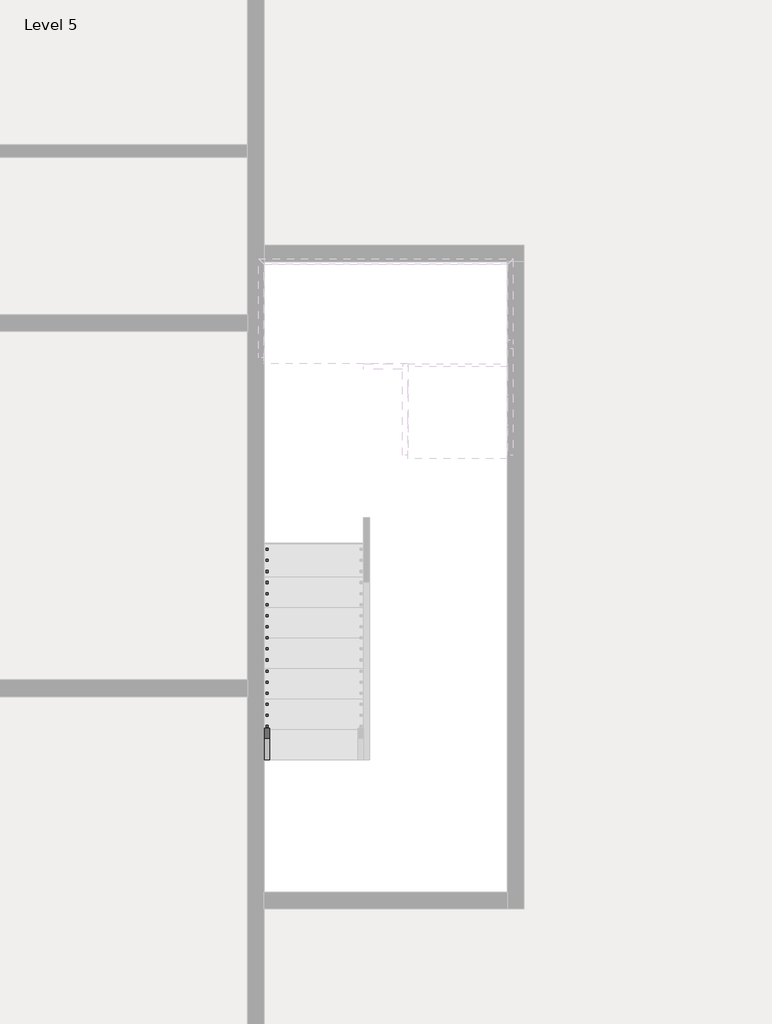
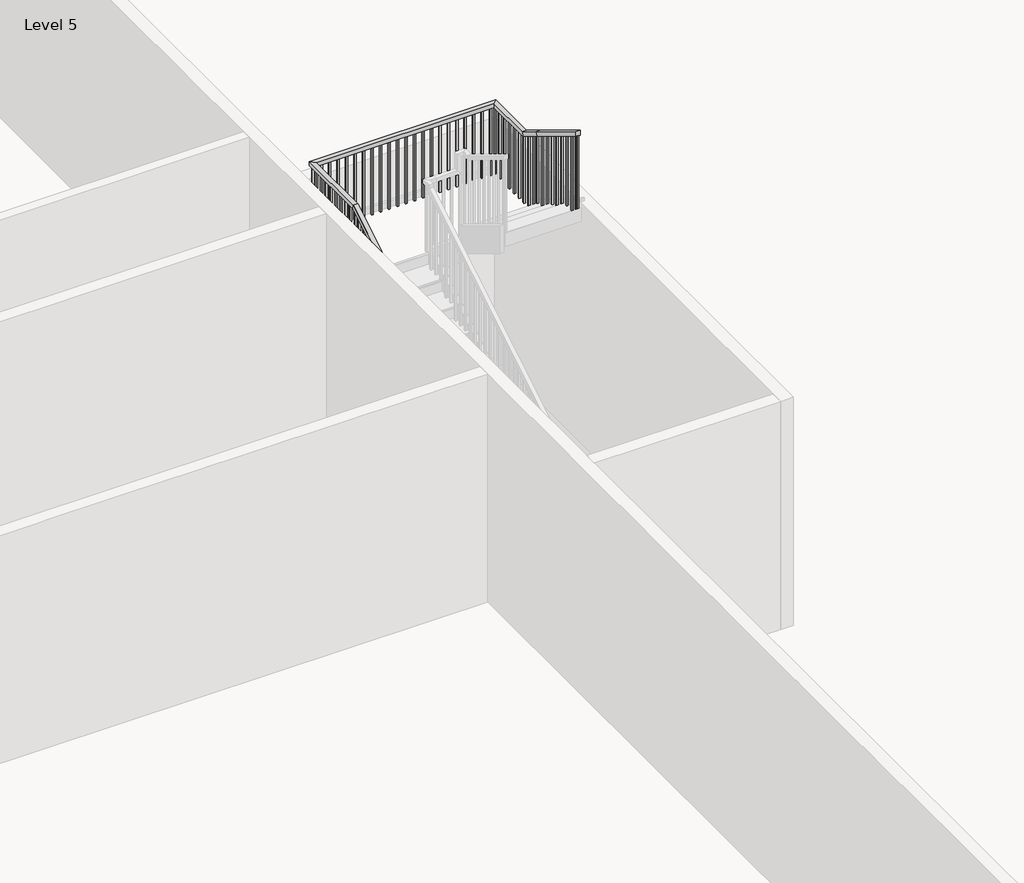
# One storey, part 6 of 8: 1 railing.
"""IFC4 building model written with IfcOpenShell, lengths in millimetres."""

from ifc_helpers import new_model, si_unit, frame, origin, place, context, project, spatial, polyline, outline, extrude, faceted_brep, element, save

model = new_model("IFC4")

# Units and contexts
model_context = context("Model", 3, world=origin())
ifc_project = project(units=[si_unit("LENGTHUNIT", "METRE", prefix="MILLI")], contexts=[model_context])

# Site, building, storey
site = spatial("IfcSite", under=ifc_project)
building = spatial("IfcBuilding", under=site)
storey = spatial("IfcBuildingStorey", under=building, Name="Level 5", Elevation=37426.6172466)

# Railing
placement = place(None, origin())
element("IfcRailing", 1, ObjectType="Handrail - Rectangular", at=placement, inside=storey, context=model_context, shape_type="SolidModel", body=[
    faceted_brep([(-3617.4415084, -23154.3851539, 38510.3505799), (-3617.4415084, -23154.3851539, 38450.9491197), (-3566.6415084, -23154.3851539, 38450.9491197), (-3566.6415084, -23154.3851539, 38510.3505799), (-3617.4415084, -19522.1851539, 40711.6839133), (-3617.4415084, -19507.9927445, 40660.8839133), (-3566.6415084, -19507.9927445, 40660.8839133), (-3566.6415084, -19522.1851539, 40711.6839133), (-3617.4415084, -18607.7851539, 40711.6839133), (-3617.4415084, -18607.7851539, 40660.8839133), (-3566.6415084, -18658.5851539, 40660.8839133), (-3566.6415084, -18658.5851539, 40711.6839133), (-1382.2415084, -18607.7851539, 40711.6839133), (-1382.2415084, -18607.7851539, 40660.8839133), (-1433.0415084, -18658.5851539, 40660.8839133), (-1433.0415084, -18658.5851539, 40711.6839133), (-1382.2415084, -19242.7851539, 40711.6839133), (-1382.2415084, -19256.9775633, 40660.8839133), (-1433.0415084, -19256.9775633, 40660.8839133), (-1433.0415084, -19242.7851539, 40711.6839133), (-1382.2415084, -19522.1851539, 40881.0172466), (-1382.2415084, -19548.5148811, 40837.5731968), (-1433.0415084, -19548.5148811, 40837.5731968), (-1433.0415084, -19522.1851539, 40881.0172466), (-1382.2415084, -20360.3851539, 41389.0172466), (-1433.0415084, -20360.3851539, 41389.0172466), (-1433.0415084, -20360.3851539, 41329.6157863), (-1382.2415084, -20360.3851539, 41329.6157863)], [[[0, 1, 2, 3]], [[1, 0, 4, 5]], [[2, 1, 5, 6]], [[3, 2, 6, 7]], [[0, 3, 7, 4]], [[5, 4, 8, 9]], [[6, 5, 9, 10]], [[7, 6, 10, 11]], [[4, 7, 11, 8]], [[9, 8, 12, 13]], [[10, 9, 13, 14]], [[11, 10, 14, 15]], [[8, 11, 15, 12]], [[13, 12, 16, 17]], [[14, 13, 17, 18]], [[15, 14, 18, 19]], [[12, 15, 19, 16]], [[17, 16, 20, 21]], [[18, 17, 21, 22]], [[19, 18, 22, 23]], [[16, 19, 23, 20]], [[24, 25, 26, 27]], [[21, 20, 24, 27]], [[22, 21, 27, 26]], [[23, 22, 26, 25]], [[20, 23, 25, 24]]]),
    extrude(outline(polyline([(-20325.4601539, 41308.4491197), (-20325.4601539, 40305.2839133), (-20344.5101539, 40305.2839133), (-20344.5101539, 41319.9945742), (-20325.4601539, 41308.4491197)])), frame((-1417.1665084, 0.0, 0.0), z_axis=(1.0, 0.0, 0.0), x_axis=(0.0, 1.0, 0.0)), (0.0, 0.0, 1.0), 19.05),
    extrude(outline(polyline([(-20223.8601539, 41246.8733621), (-20223.8601539, 40305.2839133), (-20242.9101539, 40305.2839133), (-20242.9101539, 41258.4188166), (-20223.8601539, 41246.8733621)])), frame((-1417.1665084, 0.0, 0.0), z_axis=(1.0, 0.0, 0.0), x_axis=(0.0, 1.0, 0.0)), (0.0, 0.0, 1.0), 19.05),
    extrude(outline(polyline([(-20122.2601539, 41185.2976045), (-20122.2601539, 40305.2839133), (-20141.3101539, 40305.2839133), (-20141.3101539, 41196.8430591), (-20122.2601539, 41185.2976045)])), frame((-1417.1665084, 0.0, 0.0), z_axis=(1.0, 0.0, 0.0), x_axis=(0.0, 1.0, 0.0)), (0.0, 0.0, 1.0), 19.05),
    extrude(outline(polyline([(-20020.6601539, 41123.721847), (-20020.6601539, 40135.9505799), (-20039.7101539, 40135.9505799), (-20039.7101539, 41135.2673015), (-20020.6601539, 41123.721847)])), frame((-1417.1665084, 0.0, 0.0), z_axis=(1.0, 0.0, 0.0), x_axis=(0.0, 1.0, 0.0)), (0.0, 0.0, 1.0), 19.05),
    extrude(outline(polyline([(-19919.0601539, 41062.1460894), (-19919.0601539, 40135.9505799), (-19938.1101539, 40135.9505799), (-19938.1101539, 41073.6915439), (-19919.0601539, 41062.1460894)])), frame((-1417.1665084, 0.0, 0.0), z_axis=(1.0, 0.0, 0.0), x_axis=(0.0, 1.0, 0.0)), (0.0, 0.0, 1.0), 19.05),
    extrude(outline(polyline([(-19817.4601539, 41000.5703318), (-19817.4601539, 40135.9505799), (-19836.5101539, 40135.9505799), (-19836.5101539, 41012.1157863), (-19817.4601539, 41000.5703318)])), frame((-1417.1665084, 0.0, 0.0), z_axis=(1.0, 0.0, 0.0), x_axis=(0.0, 1.0, 0.0)), (0.0, 0.0, 1.0), 19.05),
    extrude(outline(polyline([(-19715.8601539, 40938.9945742), (-19715.8601539, 39966.6172466), (-19734.9101539, 39966.6172466), (-19734.9101539, 40950.5400288), (-19715.8601539, 40938.9945742)])), frame((-1417.1665084, 0.0, 0.0), z_axis=(1.0, 0.0, 0.0), x_axis=(0.0, 1.0, 0.0)), (0.0, 0.0, 1.0), 19.05),
    extrude(outline(polyline([(-19614.2601539, 40877.4188166), (-19614.2601539, 39966.6172466), (-19633.3101539, 39966.6172466), (-19633.3101539, 40888.9642712), (-19614.2601539, 40877.4188166)])), frame((-1417.1665084, 0.0, 0.0), z_axis=(1.0, 0.0, 0.0), x_axis=(0.0, 1.0, 0.0)), (0.0, 0.0, 1.0), 19.05),
    extrude(outline(polyline([(-19436.4601539, 40769.6612409), (-19436.4601539, 39797.2839133), (-19455.5101539, 39797.2839133), (-19455.5101539, 40781.2066954), (-19436.4601539, 40769.6612409)])), frame((-1417.1665084, 0.0, 0.0), z_axis=(1.0, 0.0, 0.0), x_axis=(0.0, 1.0, 0.0)), (0.0, 0.0, 1.0), 19.05),
    extrude(outline(polyline([(-19334.8601539, 40708.0854833), (-19334.8601539, 39797.2839133), (-19353.9101539, 39797.2839133), (-19353.9101539, 40719.6309379), (-19334.8601539, 40708.0854833)])), frame((-1417.1665084, 0.0, 0.0), z_axis=(1.0, 0.0, 0.0), x_axis=(0.0, 1.0, 0.0)), (0.0, 0.0, 1.0), 19.05),
    extrude(outline(polyline([(-1398.1165084, -19233.2601539), (-1398.1165084, -19252.3101539), (-1417.1665084, -19252.3101539), (-1417.1665084, -19233.2601539), (-1398.1165084, -19233.2601539)])), frame((0.0, 0.0, 39797.2839133), z_axis=(0.0, 0.0, 1.0), x_axis=(1.0, 0.0, 0.0)), (0.0, 0.0, 1.0), 863.6),
    extrude(outline(polyline([(-1398.1165084, -19131.6601539), (-1398.1165084, -19150.7101539), (-1417.1665084, -19150.7101539), (-1417.1665084, -19131.6601539), (-1398.1165084, -19131.6601539)])), frame((0.0, 0.0, 39797.2839133), z_axis=(0.0, 0.0, 1.0), x_axis=(1.0, 0.0, 0.0)), (0.0, 0.0, 1.0), 863.6),
    extrude(outline(polyline([(-1398.1165084, -19030.0601539), (-1398.1165084, -19049.1101539), (-1417.1665084, -19049.1101539), (-1417.1665084, -19030.0601539), (-1398.1165084, -19030.0601539)])), frame((0.0, 0.0, 39797.2839133), z_axis=(0.0, 0.0, 1.0), x_axis=(1.0, 0.0, 0.0)), (0.0, 0.0, 1.0), 863.6),
    extrude(outline(polyline([(-1398.1165084, -18928.4601539), (-1398.1165084, -18947.5101539), (-1417.1665084, -18947.5101539), (-1417.1665084, -18928.4601539), (-1398.1165084, -18928.4601539)])), frame((0.0, 0.0, 39797.2839133), z_axis=(0.0, 0.0, 1.0), x_axis=(1.0, 0.0, 0.0)), (0.0, 0.0, 1.0), 863.6),
    extrude(outline(polyline([(-1398.1165084, -18826.8601539), (-1398.1165084, -18845.9101539), (-1417.1665084, -18845.9101539), (-1417.1665084, -18826.8601539), (-1398.1165084, -18826.8601539)])), frame((0.0, 0.0, 39797.2839133), z_axis=(0.0, 0.0, 1.0), x_axis=(1.0, 0.0, 0.0)), (0.0, 0.0, 1.0), 863.6),
    extrude(outline(polyline([(-1398.1165084, -18725.2601539), (-1398.1165084, -18744.3101539), (-1417.1665084, -18744.3101539), (-1417.1665084, -18725.2601539), (-1398.1165084, -18725.2601539)])), frame((0.0, 0.0, 39797.2839133), z_axis=(0.0, 0.0, 1.0), x_axis=(1.0, 0.0, 0.0)), (0.0, 0.0, 1.0), 863.6),
    extrude(outline(polyline([(-1467.9665084, -18623.6601539), (-1448.9165084, -18623.6601539), (-1448.9165084, -18642.7101539), (-1467.9665084, -18642.7101539), (-1467.9665084, -18623.6601539)])), frame((0.0, 0.0, 39797.2839133), z_axis=(0.0, 0.0, 1.0), x_axis=(1.0, 0.0, 0.0)), (0.0, 0.0, 1.0), 863.6),
    extrude(outline(polyline([(-1569.5665084, -18623.6601539), (-1550.5165084, -18623.6601539), (-1550.5165084, -18642.7101539), (-1569.5665084, -18642.7101539), (-1569.5665084, -18623.6601539)])), frame((0.0, 0.0, 39797.2839133), z_axis=(0.0, 0.0, 1.0), x_axis=(1.0, 0.0, 0.0)), (0.0, 0.0, 1.0), 863.6),
    extrude(outline(polyline([(-1671.1665084, -18623.6601539), (-1652.1165084, -18623.6601539), (-1652.1165084, -18642.7101539), (-1671.1665084, -18642.7101539), (-1671.1665084, -18623.6601539)])), frame((0.0, 0.0, 39797.2839133), z_axis=(0.0, 0.0, 1.0), x_axis=(1.0, 0.0, 0.0)), (0.0, 0.0, 1.0), 863.6),
    extrude(outline(polyline([(-1772.7665084, -18623.6601539), (-1753.7165084, -18623.6601539), (-1753.7165084, -18642.7101539), (-1772.7665084, -18642.7101539), (-1772.7665084, -18623.6601539)])), frame((0.0, 0.0, 39797.2839133), z_axis=(0.0, 0.0, 1.0), x_axis=(1.0, 0.0, 0.0)), (0.0, 0.0, 1.0), 863.6),
    extrude(outline(polyline([(-1874.3665084, -18623.6601539), (-1855.3165084, -18623.6601539), (-1855.3165084, -18642.7101539), (-1874.3665084, -18642.7101539), (-1874.3665084, -18623.6601539)])), frame((0.0, 0.0, 39797.2839133), z_axis=(0.0, 0.0, 1.0), x_axis=(1.0, 0.0, 0.0)), (0.0, 0.0, 1.0), 863.6),
    extrude(outline(polyline([(-1975.9665084, -18623.6601539), (-1956.9165084, -18623.6601539), (-1956.9165084, -18642.7101539), (-1975.9665084, -18642.7101539), (-1975.9665084, -18623.6601539)])), frame((0.0, 0.0, 39797.2839133), z_axis=(0.0, 0.0, 1.0), x_axis=(1.0, 0.0, 0.0)), (0.0, 0.0, 1.0), 863.6),
    extrude(outline(polyline([(-2077.5665084, -18623.6601539), (-2058.5165084, -18623.6601539), (-2058.5165084, -18642.7101539), (-2077.5665084, -18642.7101539), (-2077.5665084, -18623.6601539)])), frame((0.0, 0.0, 39797.2839133), z_axis=(0.0, 0.0, 1.0), x_axis=(1.0, 0.0, 0.0)), (0.0, 0.0, 1.0), 863.6),
    extrude(outline(polyline([(-2179.1665084, -18623.6601539), (-2160.1165084, -18623.6601539), (-2160.1165084, -18642.7101539), (-2179.1665084, -18642.7101539), (-2179.1665084, -18623.6601539)])), frame((0.0, 0.0, 39797.2839133), z_axis=(0.0, 0.0, 1.0), x_axis=(1.0, 0.0, 0.0)), (0.0, 0.0, 1.0), 863.6),
    extrude(outline(polyline([(-2280.7665084, -18623.6601539), (-2261.7165084, -18623.6601539), (-2261.7165084, -18642.7101539), (-2280.7665084, -18642.7101539), (-2280.7665084, -18623.6601539)])), frame((0.0, 0.0, 39797.2839133), z_axis=(0.0, 0.0, 1.0), x_axis=(1.0, 0.0, 0.0)), (0.0, 0.0, 1.0), 863.6),
    extrude(outline(polyline([(-2382.3665084, -18623.6601539), (-2363.3165084, -18623.6601539), (-2363.3165084, -18642.7101539), (-2382.3665084, -18642.7101539), (-2382.3665084, -18623.6601539)])), frame((0.0, 0.0, 39797.2839133), z_axis=(0.0, 0.0, 1.0), x_axis=(1.0, 0.0, 0.0)), (0.0, 0.0, 1.0), 863.6),
    extrude(outline(polyline([(-2483.9665084, -18623.6601539), (-2464.9165084, -18623.6601539), (-2464.9165084, -18642.7101539), (-2483.9665084, -18642.7101539), (-2483.9665084, -18623.6601539)])), frame((0.0, 0.0, 39797.2839133), z_axis=(0.0, 0.0, 1.0), x_axis=(1.0, 0.0, 0.0)), (0.0, 0.0, 1.0), 863.6),
    extrude(outline(polyline([(-2585.5665084, -18623.6601539), (-2566.5165084, -18623.6601539), (-2566.5165084, -18642.7101539), (-2585.5665084, -18642.7101539), (-2585.5665084, -18623.6601539)])), frame((0.0, 0.0, 39797.2839133), z_axis=(0.0, 0.0, 1.0), x_axis=(1.0, 0.0, 0.0)), (0.0, 0.0, 1.0), 863.6),
    extrude(outline(polyline([(-2687.1665084, -18623.6601539), (-2668.1165084, -18623.6601539), (-2668.1165084, -18642.7101539), (-2687.1665084, -18642.7101539), (-2687.1665084, -18623.6601539)])), frame((0.0, 0.0, 39797.2839133), z_axis=(0.0, 0.0, 1.0), x_axis=(1.0, 0.0, 0.0)), (0.0, 0.0, 1.0), 863.6),
    extrude(outline(polyline([(-2788.7665084, -18623.6601539), (-2769.7165084, -18623.6601539), (-2769.7165084, -18642.7101539), (-2788.7665084, -18642.7101539), (-2788.7665084, -18623.6601539)])), frame((0.0, 0.0, 39797.2839133), z_axis=(0.0, 0.0, 1.0), x_axis=(1.0, 0.0, 0.0)), (0.0, 0.0, 1.0), 863.6),
    extrude(outline(polyline([(-2890.3665084, -18623.6601539), (-2871.3165084, -18623.6601539), (-2871.3165084, -18642.7101539), (-2890.3665084, -18642.7101539), (-2890.3665084, -18623.6601539)])), frame((0.0, 0.0, 39797.2839133), z_axis=(0.0, 0.0, 1.0), x_axis=(1.0, 0.0, 0.0)), (0.0, 0.0, 1.0), 863.6),
    extrude(outline(polyline([(-2991.9665084, -18623.6601539), (-2972.9165084, -18623.6601539), (-2972.9165084, -18642.7101539), (-2991.9665084, -18642.7101539), (-2991.9665084, -18623.6601539)])), frame((0.0, 0.0, 39797.2839133), z_axis=(0.0, 0.0, 1.0), x_axis=(1.0, 0.0, 0.0)), (0.0, 0.0, 1.0), 863.6),
    extrude(outline(polyline([(-3093.5665084, -18623.6601539), (-3074.5165084, -18623.6601539), (-3074.5165084, -18642.7101539), (-3093.5665084, -18642.7101539), (-3093.5665084, -18623.6601539)])), frame((0.0, 0.0, 39797.2839133), z_axis=(0.0, 0.0, 1.0), x_axis=(1.0, 0.0, 0.0)), (0.0, 0.0, 1.0), 863.6),
    extrude(outline(polyline([(-3195.1665084, -18623.6601539), (-3176.1165084, -18623.6601539), (-3176.1165084, -18642.7101539), (-3195.1665084, -18642.7101539), (-3195.1665084, -18623.6601539)])), frame((0.0, 0.0, 39797.2839133), z_axis=(0.0, 0.0, 1.0), x_axis=(1.0, 0.0, 0.0)), (0.0, 0.0, 1.0), 863.6),
    extrude(outline(polyline([(-3296.7665084, -18623.6601539), (-3277.7165084, -18623.6601539), (-3277.7165084, -18642.7101539), (-3296.7665084, -18642.7101539), (-3296.7665084, -18623.6601539)])), frame((0.0, 0.0, 39797.2839133), z_axis=(0.0, 0.0, 1.0), x_axis=(1.0, 0.0, 0.0)), (0.0, 0.0, 1.0), 863.6),
    extrude(outline(polyline([(-3398.3665084, -18623.6601539), (-3379.3165084, -18623.6601539), (-3379.3165084, -18642.7101539), (-3398.3665084, -18642.7101539), (-3398.3665084, -18623.6601539)])), frame((0.0, 0.0, 39797.2839133), z_axis=(0.0, 0.0, 1.0), x_axis=(1.0, 0.0, 0.0)), (0.0, 0.0, 1.0), 863.6),
    extrude(outline(polyline([(-3499.9665084, -18623.6601539), (-3480.9165084, -18623.6601539), (-3480.9165084, -18642.7101539), (-3499.9665084, -18642.7101539), (-3499.9665084, -18623.6601539)])), frame((0.0, 0.0, 39797.2839133), z_axis=(0.0, 0.0, 1.0), x_axis=(1.0, 0.0, 0.0)), (0.0, 0.0, 1.0), 863.6),
    extrude(outline(polyline([(-3601.5665084, -18718.9101539), (-3601.5665084, -18699.8601539), (-3582.5165084, -18699.8601539), (-3582.5165084, -18718.9101539), (-3601.5665084, -18718.9101539)])), frame((0.0, 0.0, 39797.2839133), z_axis=(0.0, 0.0, 1.0), x_axis=(1.0, 0.0, 0.0)), (0.0, 0.0, 1.0), 863.6),
    extrude(outline(polyline([(-3601.5665084, -18820.5101539), (-3601.5665084, -18801.4601539), (-3582.5165084, -18801.4601539), (-3582.5165084, -18820.5101539), (-3601.5665084, -18820.5101539)])), frame((0.0, 0.0, 39797.2839133), z_axis=(0.0, 0.0, 1.0), x_axis=(1.0, 0.0, 0.0)), (0.0, 0.0, 1.0), 863.6),
    extrude(outline(polyline([(-3601.5665084, -18922.1101539), (-3601.5665084, -18903.0601539), (-3582.5165084, -18903.0601539), (-3582.5165084, -18922.1101539), (-3601.5665084, -18922.1101539)])), frame((0.0, 0.0, 39797.2839133), z_axis=(0.0, 0.0, 1.0), x_axis=(1.0, 0.0, 0.0)), (0.0, 0.0, 1.0), 863.6),
    extrude(outline(polyline([(-3601.5665084, -19023.7101539), (-3601.5665084, -19004.6601539), (-3582.5165084, -19004.6601539), (-3582.5165084, -19023.7101539), (-3601.5665084, -19023.7101539)])), frame((0.0, 0.0, 39797.2839133), z_axis=(0.0, 0.0, 1.0), x_axis=(1.0, 0.0, 0.0)), (0.0, 0.0, 1.0), 863.6),
    extrude(outline(polyline([(-3601.5665084, -19125.3101539), (-3601.5665084, -19106.2601539), (-3582.5165084, -19106.2601539), (-3582.5165084, -19125.3101539), (-3601.5665084, -19125.3101539)])), frame((0.0, 0.0, 39797.2839133), z_axis=(0.0, 0.0, 1.0), x_axis=(1.0, 0.0, 0.0)), (0.0, 0.0, 1.0), 863.6),
    extrude(outline(polyline([(-3601.5665084, -19226.9101539), (-3601.5665084, -19207.8601539), (-3582.5165084, -19207.8601539), (-3582.5165084, -19226.9101539), (-3601.5665084, -19226.9101539)])), frame((0.0, 0.0, 39797.2839133), z_axis=(0.0, 0.0, 1.0), x_axis=(1.0, 0.0, 0.0)), (0.0, 0.0, 1.0), 863.6),
    extrude(outline(polyline([(-3601.5665084, -19328.5101539), (-3601.5665084, -19309.4601539), (-3582.5165084, -19309.4601539), (-3582.5165084, -19328.5101539), (-3601.5665084, -19328.5101539)])), frame((0.0, 0.0, 39797.2839133), z_axis=(0.0, 0.0, 1.0), x_axis=(1.0, 0.0, 0.0)), (0.0, 0.0, 1.0), 863.6),
    extrude(outline(polyline([(-3601.5665084, -19430.1101539), (-3601.5665084, -19411.0601539), (-3582.5165084, -19411.0601539), (-3582.5165084, -19430.1101539), (-3601.5665084, -19430.1101539)])), frame((0.0, 0.0, 39797.2839133), z_axis=(0.0, 0.0, 1.0), x_axis=(1.0, 0.0, 0.0)), (0.0, 0.0, 1.0), 863.6),
    extrude(outline(polyline([(-19588.8601539, 40611.8733621), (-19588.8601539, 39627.9505799), (-19607.9101539, 39627.9505799), (-19607.9101539, 40600.3279076), (-19588.8601539, 40611.8733621)])), frame((-3601.5665084, 0.0, 0.0), z_axis=(1.0, 0.0, 0.0), x_axis=(0.0, 1.0, 0.0)), (0.0, 0.0, 1.0), 19.05),
    extrude(outline(polyline([(-19690.4601539, 40550.2976045), (-19690.4601539, 39627.9505799), (-19709.5101539, 39627.9505799), (-19709.5101539, 40538.75215), (-19690.4601539, 40550.2976045)])), frame((-3601.5665084, 0.0, 0.0), z_axis=(1.0, 0.0, 0.0), x_axis=(0.0, 1.0, 0.0)), (0.0, 0.0, 1.0), 19.05),
    extrude(outline(polyline([(-19792.0601539, 40488.721847), (-19792.0601539, 39627.9505799), (-19811.1101539, 39627.9505799), (-19811.1101539, 40477.1763924), (-19792.0601539, 40488.721847)])), frame((-3601.5665084, 0.0, 0.0), z_axis=(1.0, 0.0, 0.0), x_axis=(0.0, 1.0, 0.0)), (0.0, 0.0, 1.0), 19.05),
    extrude(outline(polyline([(-19893.6601539, 40427.1460894), (-19893.6601539, 39458.6172466), (-19912.7101539, 39458.6172466), (-19912.7101539, 40415.6006348), (-19893.6601539, 40427.1460894)])), frame((-3601.5665084, 0.0, 0.0), z_axis=(1.0, 0.0, 0.0), x_axis=(0.0, 1.0, 0.0)), (0.0, 0.0, 1.0), 19.05),
    extrude(outline(polyline([(-19995.2601539, 40365.5703318), (-19995.2601539, 39458.6172466), (-20014.3101539, 39458.6172466), (-20014.3101539, 40354.0248773), (-19995.2601539, 40365.5703318)])), frame((-3601.5665084, 0.0, 0.0), z_axis=(1.0, 0.0, 0.0), x_axis=(0.0, 1.0, 0.0)), (0.0, 0.0, 1.0), 19.05),
    extrude(outline(polyline([(-20096.8601539, 40303.9945742), (-20096.8601539, 39289.2839133), (-20115.9101539, 39289.2839133), (-20115.9101539, 40292.4491197), (-20096.8601539, 40303.9945742)])), frame((-3601.5665084, 0.0, 0.0), z_axis=(1.0, 0.0, 0.0), x_axis=(0.0, 1.0, 0.0)), (0.0, 0.0, 1.0), 19.05),
    extrude(outline(polyline([(-20198.4601539, 40242.4188166), (-20198.4601539, 39289.2839133), (-20217.5101539, 39289.2839133), (-20217.5101539, 40230.8733621), (-20198.4601539, 40242.4188166)])), frame((-3601.5665084, 0.0, 0.0), z_axis=(1.0, 0.0, 0.0), x_axis=(0.0, 1.0, 0.0)), (0.0, 0.0, 1.0), 19.05),
    extrude(outline(polyline([(-20300.0601539, 40180.8430591), (-20300.0601539, 39289.2839133), (-20319.1101539, 39289.2839133), (-20319.1101539, 40169.2976045), (-20300.0601539, 40180.8430591)])), frame((-3601.5665084, 0.0, 0.0), z_axis=(1.0, 0.0, 0.0), x_axis=(0.0, 1.0, 0.0)), (0.0, 0.0, 1.0), 19.05),
    extrude(outline(polyline([(-20401.6601539, 40119.2673015), (-20401.6601539, 39119.9505799), (-20420.7101539, 39119.9505799), (-20420.7101539, 40107.721847), (-20401.6601539, 40119.2673015)])), frame((-3601.5665084, 0.0, 0.0), z_axis=(1.0, 0.0, 0.0), x_axis=(0.0, 1.0, 0.0)), (0.0, 0.0, 1.0), 19.05),
    extrude(outline(polyline([(-20503.2601539, 40057.6915439), (-20503.2601539, 39119.9505799), (-20522.3101539, 39119.9505799), (-20522.3101539, 40046.1460894), (-20503.2601539, 40057.6915439)])), frame((-3601.5665084, 0.0, 0.0), z_axis=(1.0, 0.0, 0.0), x_axis=(0.0, 1.0, 0.0)), (0.0, 0.0, 1.0), 19.05),
    extrude(outline(polyline([(-20604.8601539, 39996.1157863), (-20604.8601539, 39119.9505799), (-20623.9101539, 39119.9505799), (-20623.9101539, 39984.5703318), (-20604.8601539, 39996.1157863)])), frame((-3601.5665084, 0.0, 0.0), z_axis=(1.0, 0.0, 0.0), x_axis=(0.0, 1.0, 0.0)), (0.0, 0.0, 1.0), 19.05),
    extrude(outline(polyline([(-20706.4601539, 39934.5400288), (-20706.4601539, 38950.6172466), (-20725.5101539, 38950.6172466), (-20725.5101539, 39922.9945742), (-20706.4601539, 39934.5400288)])), frame((-3601.5665084, 0.0, 0.0), z_axis=(1.0, 0.0, 0.0), x_axis=(0.0, 1.0, 0.0)), (0.0, 0.0, 1.0), 19.05),
    extrude(outline(polyline([(-20808.0601539, 39872.9642712), (-20808.0601539, 38950.6172466), (-20827.1101539, 38950.6172466), (-20827.1101539, 39861.4188166), (-20808.0601539, 39872.9642712)])), frame((-3601.5665084, 0.0, 0.0), z_axis=(1.0, 0.0, 0.0), x_axis=(0.0, 1.0, 0.0)), (0.0, 0.0, 1.0), 19.05),
    extrude(outline(polyline([(-20909.6601539, 39811.3885136), (-20909.6601539, 38950.6172466), (-20928.7101539, 38950.6172466), (-20928.7101539, 39799.8430591), (-20909.6601539, 39811.3885136)])), frame((-3601.5665084, 0.0, 0.0), z_axis=(1.0, 0.0, 0.0), x_axis=(0.0, 1.0, 0.0)), (0.0, 0.0, 1.0), 19.05),
    extrude(outline(polyline([(-21011.2601539, 39749.812756), (-21011.2601539, 38781.2839133), (-21030.3101539, 38781.2839133), (-21030.3101539, 39738.2673015), (-21011.2601539, 39749.812756)])), frame((-3601.5665084, 0.0, 0.0), z_axis=(1.0, 0.0, 0.0), x_axis=(0.0, 1.0, 0.0)), (0.0, 0.0, 1.0), 19.05),
    extrude(outline(polyline([(-21112.8601539, 39688.2369985), (-21112.8601539, 38781.2839133), (-21131.9101539, 38781.2839133), (-21131.9101539, 39676.6915439), (-21112.8601539, 39688.2369985)])), frame((-3601.5665084, 0.0, 0.0), z_axis=(1.0, 0.0, 0.0), x_axis=(0.0, 1.0, 0.0)), (0.0, 0.0, 1.0), 19.05),
    extrude(outline(polyline([(-21214.4601539, 39626.6612409), (-21214.4601539, 38611.9505799), (-21233.5101539, 38611.9505799), (-21233.5101539, 39615.1157863), (-21214.4601539, 39626.6612409)])), frame((-3601.5665084, 0.0, 0.0), z_axis=(1.0, 0.0, 0.0), x_axis=(0.0, 1.0, 0.0)), (0.0, 0.0, 1.0), 19.05),
    extrude(outline(polyline([(-21316.0601539, 39565.0854833), (-21316.0601539, 38611.9505799), (-21335.1101539, 38611.9505799), (-21335.1101539, 39553.5400288), (-21316.0601539, 39565.0854833)])), frame((-3601.5665084, 0.0, 0.0), z_axis=(1.0, 0.0, 0.0), x_axis=(0.0, 1.0, 0.0)), (0.0, 0.0, 1.0), 19.05),
    extrude(outline(polyline([(-21417.6601539, 39503.5097257), (-21417.6601539, 38611.9505799), (-21436.7101539, 38611.9505799), (-21436.7101539, 39491.9642712), (-21417.6601539, 39503.5097257)])), frame((-3601.5665084, 0.0, 0.0), z_axis=(1.0, 0.0, 0.0), x_axis=(0.0, 1.0, 0.0)), (0.0, 0.0, 1.0), 19.05),
    extrude(outline(polyline([(-21519.2601539, 39441.9339682), (-21519.2601539, 38442.6172466), (-21538.3101539, 38442.6172466), (-21538.3101539, 39430.3885136), (-21519.2601539, 39441.9339682)])), frame((-3601.5665084, 0.0, 0.0), z_axis=(1.0, 0.0, 0.0), x_axis=(0.0, 1.0, 0.0)), (0.0, 0.0, 1.0), 19.05),
    extrude(outline(polyline([(-21620.8601539, 39380.3582106), (-21620.8601539, 38442.6172466), (-21639.9101539, 38442.6172466), (-21639.9101539, 39368.812756), (-21620.8601539, 39380.3582106)])), frame((-3601.5665084, 0.0, 0.0), z_axis=(1.0, 0.0, 0.0), x_axis=(0.0, 1.0, 0.0)), (0.0, 0.0, 1.0), 19.05),
    extrude(outline(polyline([(-21722.4601539, 39318.782453), (-21722.4601539, 38442.6172466), (-21741.5101539, 38442.6172466), (-21741.5101539, 39307.2369985), (-21722.4601539, 39318.782453)])), frame((-3601.5665084, 0.0, 0.0), z_axis=(1.0, 0.0, 0.0), x_axis=(0.0, 1.0, 0.0)), (0.0, 0.0, 1.0), 19.05),
    extrude(outline(polyline([(-21824.0601539, 39257.2066954), (-21824.0601539, 38273.2839133), (-21843.1101539, 38273.2839133), (-21843.1101539, 39245.6612409), (-21824.0601539, 39257.2066954)])), frame((-3601.5665084, 0.0, 0.0), z_axis=(1.0, 0.0, 0.0), x_axis=(0.0, 1.0, 0.0)), (0.0, 0.0, 1.0), 19.05),
    extrude(outline(polyline([(-21925.6601539, 39195.6309379), (-21925.6601539, 38273.2839133), (-21944.7101539, 38273.2839133), (-21944.7101539, 39184.0854833), (-21925.6601539, 39195.6309379)])), frame((-3601.5665084, 0.0, 0.0), z_axis=(1.0, 0.0, 0.0), x_axis=(0.0, 1.0, 0.0)), (0.0, 0.0, 1.0), 19.05),
    extrude(outline(polyline([(-22027.2601539, 39134.0551803), (-22027.2601539, 38273.2839133), (-22046.3101539, 38273.2839133), (-22046.3101539, 39122.5097257), (-22027.2601539, 39134.0551803)])), frame((-3601.5665084, 0.0, 0.0), z_axis=(1.0, 0.0, 0.0), x_axis=(0.0, 1.0, 0.0)), (0.0, 0.0, 1.0), 19.05),
    extrude(outline(polyline([(-22128.8601539, 39072.4794227), (-22128.8601539, 38103.9505799), (-22147.9101539, 38103.9505799), (-22147.9101539, 39060.9339682), (-22128.8601539, 39072.4794227)])), frame((-3601.5665084, 0.0, 0.0), z_axis=(1.0, 0.0, 0.0), x_axis=(0.0, 1.0, 0.0)), (0.0, 0.0, 1.0), 19.05),
    extrude(outline(polyline([(-22230.4601539, 39010.9036651), (-22230.4601539, 38103.9505799), (-22249.5101539, 38103.9505799), (-22249.5101539, 38999.3582106), (-22230.4601539, 39010.9036651)])), frame((-3601.5665084, 0.0, 0.0), z_axis=(1.0, 0.0, 0.0), x_axis=(0.0, 1.0, 0.0)), (0.0, 0.0, 1.0), 19.05),
    extrude(outline(polyline([(-22332.0601539, 38949.3279076), (-22332.0601539, 37934.6172466), (-22351.1101539, 37934.6172466), (-22351.1101539, 38937.782453), (-22332.0601539, 38949.3279076)])), frame((-3601.5665084, 0.0, 0.0), z_axis=(1.0, 0.0, 0.0), x_axis=(0.0, 1.0, 0.0)), (0.0, 0.0, 1.0), 19.05),
    extrude(outline(polyline([(-22433.6601539, 38887.75215), (-22433.6601539, 37934.6172466), (-22452.7101539, 37934.6172466), (-22452.7101539, 38876.2066954), (-22433.6601539, 38887.75215)])), frame((-3601.5665084, 0.0, 0.0), z_axis=(1.0, 0.0, 0.0), x_axis=(0.0, 1.0, 0.0)), (0.0, 0.0, 1.0), 19.05),
    extrude(outline(polyline([(-22535.2601539, 38826.1763924), (-22535.2601539, 37934.6172466), (-22554.3101539, 37934.6172466), (-22554.3101539, 38814.6309379), (-22535.2601539, 38826.1763924)])), frame((-3601.5665084, 0.0, 0.0), z_axis=(1.0, 0.0, 0.0), x_axis=(0.0, 1.0, 0.0)), (0.0, 0.0, 1.0), 19.05),
    extrude(outline(polyline([(-22636.8601539, 38764.6006348), (-22636.8601539, 37765.2839133), (-22655.9101539, 37765.2839133), (-22655.9101539, 38753.0551803), (-22636.8601539, 38764.6006348)])), frame((-3601.5665084, 0.0, 0.0), z_axis=(1.0, 0.0, 0.0), x_axis=(0.0, 1.0, 0.0)), (0.0, 0.0, 1.0), 19.05),
    extrude(outline(polyline([(-22738.4601539, 38703.0248773), (-22738.4601539, 37765.2839133), (-22757.5101539, 37765.2839133), (-22757.5101539, 38691.4794227), (-22738.4601539, 38703.0248773)])), frame((-3601.5665084, 0.0, 0.0), z_axis=(1.0, 0.0, 0.0), x_axis=(0.0, 1.0, 0.0)), (0.0, 0.0, 1.0), 19.05),
    extrude(outline(polyline([(-22840.0601539, 38641.4491197), (-22840.0601539, 37765.2839133), (-22859.1101539, 37765.2839133), (-22859.1101539, 38629.9036651), (-22840.0601539, 38641.4491197)])), frame((-3601.5665084, 0.0, 0.0), z_axis=(1.0, 0.0, 0.0), x_axis=(0.0, 1.0, 0.0)), (0.0, 0.0, 1.0), 19.05),
    extrude(outline(polyline([(-22941.6601539, 38579.8733621), (-22941.6601539, 37595.9505799), (-22960.7101539, 37595.9505799), (-22960.7101539, 38568.3279076), (-22941.6601539, 38579.8733621)])), frame((-3601.5665084, 0.0, 0.0), z_axis=(1.0, 0.0, 0.0), x_axis=(0.0, 1.0, 0.0)), (0.0, 0.0, 1.0), 19.05),
    extrude(outline(polyline([(-23043.2601539, 38518.2976045), (-23043.2601539, 37595.9505799), (-23062.3101539, 37595.9505799), (-23062.3101539, 38506.75215), (-23043.2601539, 38518.2976045)])), frame((-3601.5665084, 0.0, 0.0), z_axis=(1.0, 0.0, 0.0), x_axis=(0.0, 1.0, 0.0)), (0.0, 0.0, 1.0), 19.05),
    extrude(outline(polyline([(-19512.6601539, 40815.8430591), (-19512.6601539, 39797.2839133), (-19531.7101539, 39797.2839133), (-19531.7101539, 40827.3885136), (-19512.6601539, 40815.8430591)])), frame((-1417.1665084, 0.0, 0.0), z_axis=(1.0, 0.0, 0.0), x_axis=(0.0, 1.0, 0.0)), (0.0, 0.0, 1.0), 19.05),
    extrude(outline(polyline([(-1417.1665084, -18623.6601539), (-1398.1165084, -18623.6601539), (-1398.1165084, -18642.7101539), (-1417.1665084, -18642.7101539), (-1417.1665084, -18623.6601539)])), frame((0.0, 0.0, 39797.2839133), z_axis=(0.0, 0.0, 1.0), x_axis=(1.0, 0.0, 0.0)), (0.0, 0.0, 1.0), 863.6),
    extrude(outline(polyline([(-3601.5665084, -18642.7101539), (-3601.5665084, -18623.6601539), (-3582.5165084, -18623.6601539), (-3582.5165084, -18642.7101539), (-3601.5665084, -18642.7101539)])), frame((0.0, 0.0, 39797.2839133), z_axis=(0.0, 0.0, 1.0), x_axis=(1.0, 0.0, 0.0)), (0.0, 0.0, 1.0), 863.6),
    extrude(outline(polyline([(-19512.6601539, 40658.0551803), (-19512.6601539, 39797.2839133), (-19531.7101539, 39797.2839133), (-19531.7101539, 40646.5097257), (-19512.6601539, 40658.0551803)])), frame((-3601.5665084, 0.0, 0.0), z_axis=(1.0, 0.0, 0.0), x_axis=(0.0, 1.0, 0.0)), (0.0, 0.0, 1.0), 19.05),
    extrude(outline(polyline([(-20341.3351539, 41318.0703318), (-20341.3351539, 40305.2839133), (-20360.3851539, 40305.2839133), (-20360.3851539, 41329.6157863), (-20341.3351539, 41318.0703318)])), frame((-1417.1665084, 0.0, 0.0), z_axis=(1.0, 0.0, 0.0), x_axis=(0.0, 1.0, 0.0)), (0.0, 0.0, 1.0), 19.05),
    extrude(outline(polyline([(-23135.3351539, 38462.4945742), (-23135.3351539, 37595.9505799), (-23154.3851539, 37595.9505799), (-23154.3851539, 38450.9491197), (-23135.3351539, 38462.4945742)])), frame((-3601.5665084, 0.0, 0.0), z_axis=(1.0, 0.0, 0.0), x_axis=(0.0, 1.0, 0.0)), (0.0, 0.0, 1.0), 19.05),
])

save(model, "model.ifc")

# Revit data of these elements
# Type "Handrail - Rectangular"
#   Assembly Code = "C2010400"
#   built-in parameter 1008612 = 0.0416667 (stored number, unit not read)
#   built-in parameter 1008611 = 0.0416667 (stored number, unit not read)
#   built-in parameter 1008609 = 0.333333 (stored number, unit not read)
#   built-in parameter 1008604 = 0.166667 (stored number, unit not read)
#   built-in parameter 1008603 = 0.166667 (stored number, unit not read)
#   Railing Height = 3' - 0"
#   built-in parameter 1008630 = 2
#   built-in parameter 1008610 = 2
#   built-in parameter 1008618 = Baluster - Square : 3/4"
# Element 1 (IfcRailing, "Handrail - Rectangular")
#   Phase Created = New Construction
